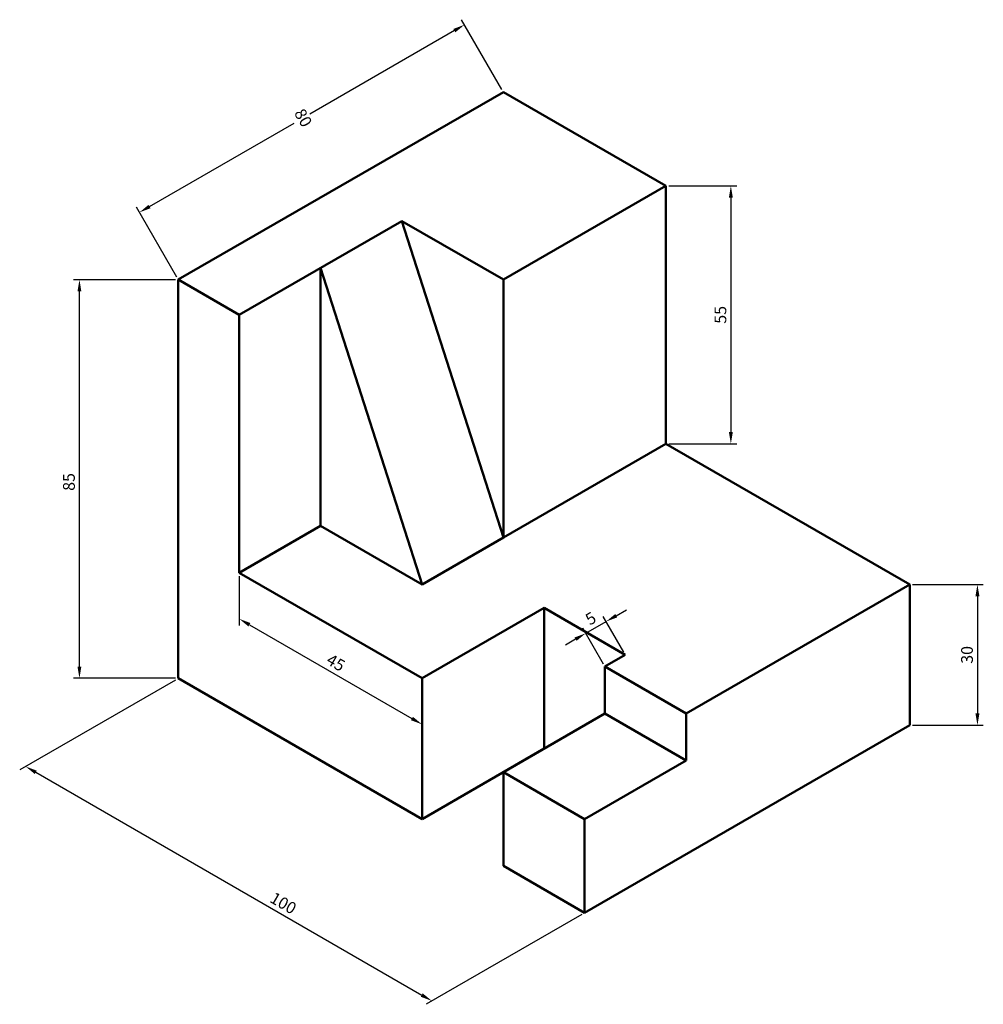
# Model space of a CAD drawing. Units: millimetres. Extents: x 2117 to 2323, y 1175 to 1385.
import ezdxf

# ---------------------------------------------------------------- set-up
doc = ezdxf.new("R2010")
doc.units = ezdxf.units.MM
doc.layers.add('M-DIMS', color=2, linetype='Continuous', lineweight=25)
doc.layers.add('M-OUTL', color=7, linetype='Continuous', lineweight=50)
doc.styles.get("Standard").update_dxf_attribs({"font": 'arial.ttf'})
doc.dimstyles.new('ISO-25', dxfattribs={"dimtxt": 2.5, "dimasz": 2.5, "dimexe": 1.25, "dimexo": 0.625, "dimtad": 1, "dimtxsty": 'Standard', "dimcen": 2.5, "dimadec": 0, "dimazin": 0, "dimtfac": 1, "dimtmove": 0, "dimatfit": 3, "dimfxl": 1, "dimarcsym": 0})

# ---------------------------------------------------------------- blocks, each defined once
blk = doc.blocks.new('*D1')
at = {"layer": 'Defpoints', "color": 0, "transparency": 16777216}
for p in [(2151.04, 1244.73), (2237.64, 1194.73), (2205.09, 1175.94)]:
    blk.add_point(p, dxfattribs=at)
at = {"layer": 'M-DIMS', "color": 0, "lineweight": -2, "transparency": 16777216}
for p, q in [((2150.41, 1244.37), (2117.24, 1225.22)), ((2120.65, 1224.69), (2202.93, 1177.19)), ((2237.01, 1194.37), (2203.84, 1175.22))]:
    blk.add_line(p, q, dxfattribs=at)
at = {"layer": 'M-DIMS', "color": 0, "transparency": 16777216}
for points in [[(2120.86, 1225.05), (2120.45, 1224.33), (2118.49, 1225.94)], [(2203.13, 1177.55), (2202.72, 1176.83), (2205.09, 1175.94)]]:
    blk.add_solid(points, dxfattribs=at)
at = {"layer": 'M-DIMS', "color": 0, "transparency": 16777216, "insert": (2173.26, 1196.52), "char_height": 2.5, "attachment_point": 5, "rotation": 330}
blk.add_mtext('100', dxfattribs=at)
blk = doc.blocks.new('*D2')
at = {"layer": 'Defpoints', "color": 0, "transparency": 16777216}
for p in [(2129.97, 1329.73), (2151.04, 1329.73), (2151.04, 1244.73)]:
    blk.add_point(p, dxfattribs=at)
at = {"layer": 'M-DIMS', "color": 0, "lineweight": -2, "transparency": 16777216}
for p, q in [((2150.41, 1329.73), (2128.72, 1329.73)), ((2129.97, 1247.23), (2129.97, 1327.23)), ((2150.41, 1244.73), (2128.72, 1244.73))]:
    blk.add_line(p, q, dxfattribs=at)
at = {"layer": 'M-DIMS', "color": 0, "transparency": 16777216}
for points in [[(2129.55, 1327.23), (2130.38, 1327.23), (2129.97, 1329.73)], [(2129.55, 1247.23), (2130.38, 1247.23), (2129.97, 1244.73)]]:
    blk.add_solid(points, dxfattribs=at)
at = {"layer": 'M-DIMS', "color": 0, "transparency": 16777216, "insert": (2128.06, 1286.6), "char_height": 2.5, "attachment_point": 5, "rotation": 90}
blk.add_mtext('85', dxfattribs=at)
blk = doc.blocks.new('*D3')
at = {"layer": 'Defpoints', "color": 0, "transparency": 16777216}
for p in [(2212.03, 1384.08), (2220.32, 1369.73), (2151.04, 1329.73)]:
    blk.add_point(p, dxfattribs=at)
at = {"layer": 'M-DIMS', "color": 0, "lineweight": -2, "transparency": 16777216}
for p, q in [((2220, 1370.28), (2211.41, 1385.17)), ((2209.87, 1382.83), (2179.04, 1365.03)), ((2144.92, 1345.33), (2175.75, 1363.13)), ((2150.72, 1330.28), (2142.13, 1345.17))]:
    blk.add_line(p, q, dxfattribs=at)
at = {"layer": 'M-DIMS', "color": 0, "transparency": 16777216}
for points in [[(2209.66, 1383.19), (2210.08, 1382.47), (2212.03, 1384.08)], [(2144.71, 1345.69), (2145.12, 1344.97), (2142.75, 1344.08)]]:
    blk.add_solid(points, dxfattribs=at)
at = {"layer": 'M-DIMS', "color": 0, "transparency": 16777216, "insert": (2177.39, 1364.08), "char_height": 2.5, "attachment_point": 5, "rotation": 300}
blk.add_mtext('80', dxfattribs=at)
blk = doc.blocks.new('*D12')
at = {"layer": 'Defpoints', "color": 0, "transparency": 16777216}
for p in [(2254.96, 1349.73), (2254.96, 1294.73), (2268.8, 1294.73)]:
    blk.add_point(p, dxfattribs=at)
at = {"layer": 'M-DIMS', "color": 0, "lineweight": -2, "transparency": 16777216}
for p, q in [((2255.58, 1349.73), (2270.05, 1349.73)), ((2268.8, 1347.23), (2268.8, 1297.23)), ((2255.58, 1294.73), (2270.05, 1294.73))]:
    blk.add_line(p, q, dxfattribs=at)
at = {"layer": 'M-DIMS', "color": 0, "transparency": 16777216}
for points in [[(2268.38, 1347.23), (2269.22, 1347.23), (2268.8, 1349.73)], [(2268.38, 1297.23), (2269.22, 1297.23), (2268.8, 1294.73)]]:
    blk.add_solid(points, dxfattribs=at)
at = {"layer": 'M-DIMS', "color": 0, "transparency": 16777216, "insert": (2266.9, 1322.23), "char_height": 2.5, "attachment_point": 5, "rotation": 90}
blk.add_mtext('55', dxfattribs=at)
blk = doc.blocks.new('*D13')
at = {"layer": 'Defpoints', "color": 0, "transparency": 16777216}
for p in [(2306.92, 1264.73), (2306.92, 1234.73), (2321.35, 1234.73)]:
    blk.add_point(p, dxfattribs=at)
at = {"layer": 'M-DIMS', "color": 0, "lineweight": -2, "transparency": 16777216}
for p, q in [((2307.54, 1264.73), (2322.6, 1264.73)), ((2321.35, 1262.23), (2321.35, 1237.23)), ((2307.54, 1234.73), (2322.6, 1234.73))]:
    blk.add_line(p, q, dxfattribs=at)
at = {"layer": 'M-DIMS', "color": 0, "transparency": 16777216}
for points in [[(2320.93, 1262.23), (2321.77, 1262.23), (2321.35, 1264.73)], [(2320.93, 1237.23), (2321.77, 1237.23), (2321.35, 1234.73)]]:
    blk.add_solid(points, dxfattribs=at)
at = {"layer": 'M-DIMS', "color": 0, "transparency": 16777216, "insert": (2319.45, 1249.73), "char_height": 2.5, "attachment_point": 5, "rotation": 90}
blk.add_mtext('30', dxfattribs=at)
blk = doc.blocks.new('*D14')
at = {"layer": 'Defpoints', "color": 0, "transparency": 16777216}
for p in [(2242.2, 1256.83), (2246.3, 1249.73), (2241.97, 1247.23)]:
    blk.add_point(p, dxfattribs=at)
at = {"layer": 'M-DIMS', "color": 0, "lineweight": -2, "transparency": 16777216}
for p, q in [((2245.99, 1250.28), (2241.58, 1257.91)), ((2244.37, 1258.08), (2246.53, 1259.33)), ((2237.87, 1254.33), (2242.2, 1256.83)), ((2241.66, 1247.78), (2237.25, 1255.41)), ((2235.71, 1253.08), (2233.54, 1251.83))]:
    blk.add_line(p, q, dxfattribs=at)
at = {"layer": 'M-DIMS', "color": 0, "transparency": 16777216}
for points in [[(2244.16, 1258.44), (2244.58, 1257.72), (2242.2, 1256.83)], [(2235.5, 1253.44), (2235.92, 1252.72), (2237.87, 1254.33)]]:
    blk.add_solid(points, dxfattribs=at)
at = {"layer": 'M-DIMS', "color": 0, "transparency": 16777216, "insert": (2239.09, 1257.22), "char_height": 2.5, "attachment_point": 5, "rotation": 30}
blk.add_mtext('5', dxfattribs=at)
blk = doc.blocks.new('*D15')
at = {"layer": 'Defpoints', "color": 0, "transparency": 16777216}
for p in [(2164.03, 1267.23), (2203, 1244.73), (2203, 1234.91)]:
    blk.add_point(p, dxfattribs=at)
at = {"layer": 'M-DIMS', "color": 0, "lineweight": -2, "transparency": 16777216}
for p, q in [((2164.03, 1266.51), (2164.03, 1255.96)), ((2166.19, 1256.16), (2200.83, 1236.16)), ((2203, 1244.01), (2203, 1233.46))]:
    blk.add_line(p, q, dxfattribs=at)
at = {"layer": 'M-DIMS', "color": 0, "transparency": 16777216}
for points in [[(2166.4, 1256.52), (2165.98, 1255.8), (2164.03, 1257.41)], [(2201.04, 1236.52), (2200.62, 1235.8), (2203, 1234.91)]]:
    blk.add_solid(points, dxfattribs=at)
at = {"layer": 'M-DIMS', "color": 0, "transparency": 16777216, "insert": (2184.46, 1247.8), "char_height": 2.5, "attachment_point": 5, "rotation": 330}
blk.add_mtext('45', dxfattribs=at)

msp = doc.modelspace()

# ---------------------------------------------------------------- linework, layer by layer
at = {"layer": 'M-OUTL'}
for p, q in [((2151.035, 1329.734), (2220.317, 1369.734)), ((2220.317, 1369.734), (2254.958, 1349.734)), ((2254.958, 1349.734), (2220.317, 1329.734)), ((2254.958, 1294.734), (2254.958, 1349.734)), ((2198.666, 1342.234), (2164.025, 1322.234)), ((2220.317, 1329.734), (2198.666, 1342.234)), ((2198.666, 1342.234), (2220.317, 1274.734)), ((2181.346, 1332.234), (2202.997, 1264.734)), ((2181.346, 1277.234), (2181.346, 1332.234)), ((2151.035, 1244.734), (2151.035, 1329.734)), ((2164.025, 1322.234), (2151.035, 1329.734)), ((2220.317, 1274.734), (2220.317, 1329.734)), ((2164.025, 1322.234), (2164.025, 1267.234)), ((2254.958, 1294.734), (2220.317, 1274.734)), ((2306.92, 1264.734), (2254.958, 1294.734)), ((2164.025, 1267.234), (2181.346, 1277.234)), ((2181.346, 1277.234), (2202.997, 1264.734)), ((2220.317, 1274.734), (2202.997, 1264.734)), ((2164.025, 1267.234), (2202.997, 1244.734)), ((2259.288, 1237.234), (2306.92, 1264.734)), ((2306.92, 1264.734), (2306.92, 1234.734)), ((2202.997, 1244.734), (2228.977, 1259.734)), ((2228.977, 1259.734), (2246.298, 1249.734)), ((2228.977, 1229.734), (2228.977, 1259.734)), ((2246.298, 1249.734), (2241.968, 1247.234)), ((2241.968, 1247.234), (2259.288, 1237.234)), ((2241.968, 1237.234), (2241.968, 1247.234)), ((2151.035, 1244.734), (2202.997, 1214.734)), ((2202.997, 1214.734), (2202.997, 1244.734)), ((2220.317, 1224.734), (2241.968, 1237.234)), ((2241.968, 1237.234), (2259.288, 1227.234)), ((2259.288, 1227.234), (2259.288, 1237.234)), ((2306.92, 1234.734), (2237.638, 1194.734)), ((2202.997, 1214.734), (2228.977, 1229.734)), ((2237.638, 1214.734), (2259.288, 1227.234)), ((2220.317, 1204.734), (2220.317, 1224.734)), ((2220.317, 1224.734), (2237.638, 1214.734)), ((2237.638, 1194.734), (2237.638, 1214.734)), ((2237.638, 1194.734), (2220.317, 1204.734))]:
    msp.add_line(p, q, dxfattribs=at)

# ---------------------------------------------------------------- dimensions: what is measured, and where the dimension line sits
at = {"layer": 'M-DIMS'}
dim = msp.add_aligned_dim(p1=(2151.035, 1329.734), p2=(2220.317, 1369.734), distance=16.568, dimstyle='ISO-25', override={"dimclrd": 0, "dimclre": 0, "dimclrt": 0}, dxfattribs=at)
dim.commit()
dim.dimension.update_dxf_attribs({"geometry": '*D3', "text_midpoint": (2177.392, 1364.083), "text_rotation": 300})
for p1, p2, distance, picture, middle in [((2254.958, 1349.734), (2254.958, 1294.734), 13.84, '*D12', (2266.902, 1322.234)), ((2164.025, 1267.234), (2202.997, 1244.734), -8.512, '*D15', (2184.459, 1247.798)), ((2306.92, 1264.734), (2306.92, 1234.734), 14.429, '*D13', (2319.446, 1249.734)), ((2241.968, 1247.234), (2246.298, 1249.734), 8.189, '*D14', (2239.09, 1257.219))]:
    dim = msp.add_aligned_dim(p1=p1, p2=p2, distance=distance, dimstyle='ISO-25', override={"dimclrd": 0, "dimclre": 0, "dimclrt": 0}, dxfattribs=at)
    dim.commit()
    dim.dimension.update_dxf_attribs({"geometry": picture, "text_midpoint": middle})
for base, p2, angle, picture, middle, dimtype in [((2129.965, 1329.734), (2151.035, 1329.734), 90, '*D2', (2129.965, 1286.597), 160), ((2205.092, 1175.944), (2237.638, 1194.734), 330, '*D1', (2172.312, 1194.869), 161)]:
    dim = msp.add_linear_dim(base=base, p1=(2151.035, 1244.734), p2=p2, angle=angle, dimstyle='ISO-25', override={"dimclrd": 0, "dimclre": 0, "dimclrt": 0}, dxfattribs=at)
    dim.commit()
    dim.dimension.update_dxf_attribs({"geometry": picture, "text_midpoint": middle, "dimtype": dimtype})

doc.saveas('drawing.dxf')
